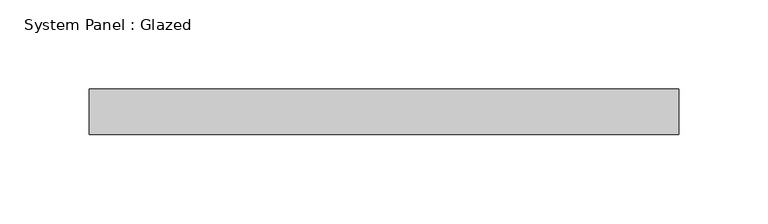
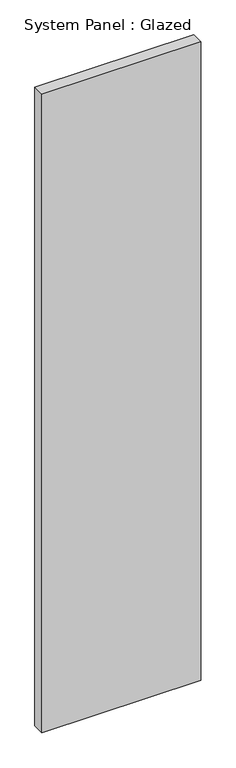
"""IFC4 building model written with IfcOpenShell, lengths in millimetres: plate geometry, System Panel : Glazed."""

from ifc_helpers import new_model, si_unit, origin, origin_with_axes, place, context, project, spatial, polyline, outline, extrude, source, transform, mapped, element, save


def system_panel_glazed_4b443884(model_context):
    return source(origin(), model_context, "Body", "SweptSolid", [
        extrude(outline(polyline([(165.1, 19.05), (-165.1, 19.05), (-165.1, 44.45), (165.1, 44.45), (165.1, 19.05)])), origin_with_axes(), (0.0, 0.0, 1.0), 1405.0284144),
    ])


if __name__ == "__main__":
    model = new_model("IFC4")
    model_context = context("Model", 3, world=origin())
    ifc_project = project(units=[si_unit("LENGTHUNIT", "METRE", prefix="MILLI")], contexts=[model_context])
    site = spatial("IfcSite", under=ifc_project)
    building = spatial("IfcBuilding", under=site)
    placement = place(None, origin())
    system_panel_glazed_shape = system_panel_glazed_4b443884(model_context)
    element("IfcPlate", 1, ObjectType="System Panel : Glazed", at=placement, inside=building, context=model_context, shape_type="MappedRepresentation", body=[
        mapped(system_panel_glazed_shape, transform((0.0, 0.0, 0.0), x_axis=(1.0, 0.0, 0.0), y_axis=(0.0, 1.0, 0.0), z_axis=(0.0, 0.0, 1.0))),
    ])
    save(model, "model.ifc")

# Revit data of these elements
# Type "System Panel : Glazed"
#   Construction Type Id = "GSP4R"
#   Analytic Construction = "1/8 in Pilkington single glazing"
#   Visual Light Transmittance = 0.9
#   Solar Heat Gain Coefficient = 0.86
#   Heat Transfer Coefficient (U) = 1.18115 BTU/(h·ft²·°F)
#   Define Thermal Properties by = 1
# Element 1 (IfcPlate, "System Panel : Glazed")
#   Materials on its faces: "Glass"
# Materials
#   "Glass": class "Glass", colour RGB 0 128 192, transparency 0.75, Description = "Soda Lime Glass", Cost = 0
